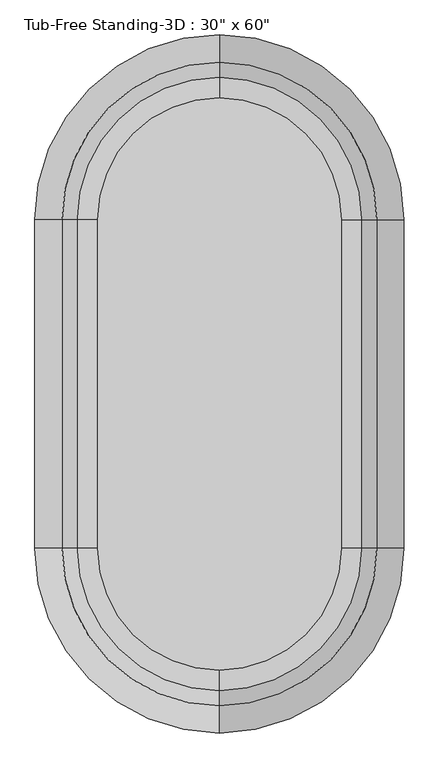
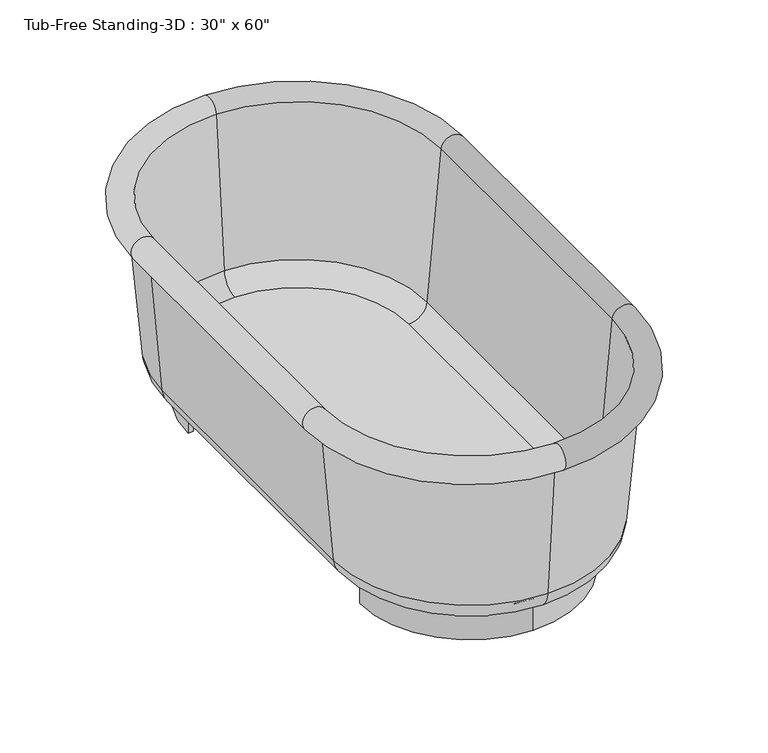
"""IFC4 building model written with IfcOpenShell, lengths in millimetres: flow terminal geometry."""

from ifc_helpers import new_model, si_unit, point, frame, frame_2d, origin, origin_with_axes, place, context, project, spatial, polyline, circle_curve, ellipse_curve, trimmed, segment, composite_curve, outline, extrude, source, transform, mapped, element, save
from ifc_brep_helpers import plane_surface, cylinder_surface, revolved_surface, advanced_brep


def flow_terminal_93af9e75(model_context):
    return source(origin(), model_context, "Body", "SolidModel", [
        extrude(outline(composite_curve([segment(trimmed(circle_curve(frame_2d((0.0, 304.8)), 215.9), [point((0.0, 520.7))], [point((-215.9, 304.8))], True, "CARTESIAN"), True, "CONTINUOUS"), segment(polyline([(-215.9, 304.8), (-226.1824236, 304.8)]), True, "CONTINUOUS"), segment(trimmed(circle_curve(frame_2d((0.0, 304.8)), 226.1824236), [point((-226.1824236, 304.8))], [point((0.0, 530.9824236))], False, "CARTESIAN"), True, "CONTINUOUS"), segment(trimmed(circle_curve(frame_2d((0.0, 304.8)), 226.1824236), [point((0.0, 530.9824236))], [point((226.1824236, 304.8))], False, "CARTESIAN"), True, "CONTINUOUS"), segment(polyline([(226.1824236, 304.8), (215.9, 304.8)]), True, "CONTINUOUS"), segment(trimmed(circle_curve(frame_2d((0.0, 304.8)), 215.9), [point((215.9, 304.8))], [point((0.0, 520.7))], True, "CARTESIAN"), True, "CONTINUOUS")], self_intersect=False)), origin_with_axes(), (0.0, 0.0, 1.0), 63.5),
        extrude(outline(composite_curve([segment(trimmed(circle_curve(frame_2d((0.0, -304.8)), 226.1824236), [point((0.0, -530.9824236))], [point((-226.1824236, -304.8))], False, "CARTESIAN"), True, "CONTINUOUS"), segment(polyline([(-226.1824236, -304.8), (-215.9, -304.8)]), True, "CONTINUOUS"), segment(trimmed(circle_curve(frame_2d((0.0, -304.8)), 215.9), [point((-215.9, -304.8))], [point((0.0, -520.7))], True, "CARTESIAN"), True, "CONTINUOUS"), segment(trimmed(circle_curve(frame_2d((0.0, -304.8)), 215.9), [point((0.0, -520.7))], [point((215.9, -304.8))], True, "CARTESIAN"), True, "CONTINUOUS"), segment(polyline([(215.9, -304.8), (226.1824236, -304.8)]), True, "CONTINUOUS"), segment(trimmed(circle_curve(frame_2d((0.0, -304.8)), 226.1824236), [point((226.1824236, -304.8))], [point((0.0, -530.9824236))], False, "CARTESIAN"), True, "CONTINUOUS")], self_intersect=False)), origin_with_axes(), (0.0, 0.0, 1.0), 63.5),
        extrude(outline(composite_curve([segment(polyline([(-226.1824236, -304.8), (-226.1824236, 304.8)]), True, "CONTINUOUS"), segment(trimmed(circle_curve(frame_2d((0.0, 304.8)), 226.1824236), [point((-226.1824236, 304.8))], [point((0.0, 530.9824236))], False, "CARTESIAN"), True, "CONTINUOUS"), segment(trimmed(circle_curve(frame_2d((0.0, 304.8)), 226.1824236), [point((0.0, 530.9824236))], [point((226.1824236, 304.8))], False, "CARTESIAN"), True, "CONTINUOUS"), segment(polyline([(226.1824236, 304.8), (226.1824236, -304.8)]), True, "CONTINUOUS"), segment(trimmed(circle_curve(frame_2d((0.0, -304.8)), 226.1824236), [point((226.1824236, -304.8))], [point((0.0, -530.9824236))], False, "CARTESIAN"), True, "CONTINUOUS"), segment(trimmed(circle_curve(frame_2d((0.0, -304.8)), 226.1824236), [point((0.0, -530.9824236))], [point((-226.1824236, -304.8))], False, "CARTESIAN"), True, "CONTINUOUS")], self_intersect=False)), frame((0.0, 0.0, 63.5), z_axis=(0.0, 0.0, 1.0), x_axis=(1.0, 0.0, 0.0)), (0.0, 0.0, 1.0), 15.08125),
        advanced_brep(
        [(0.0, -609.6, 406.4), (304.8, -304.8, 406.4), (317.5, -304.8, 406.4), (0.0, -622.3, 406.4), (0.0, -583.8045038, 111.5561295), (279.0045038, -304.8, 111.5561295), (0.0, -530.9824236, 63.1536107), (226.1824236, -304.8, 63.1536107), (0.0, -530.9824236, 78.0774627), (226.1824236, -304.8, 78.0774627), (0.0, -568.9374416, 112.8568289), (264.1374416, -304.8, 112.8568289), (0.0, -597.1561556, 435.3982063), (292.3561556, -304.8, 435.3982063), (-304.8, -304.8, 406.4), (-317.5, -304.8, 406.4), (-279.0045038, -304.8, 111.5561295), (-226.1824236, -304.8, 63.1536107), (-226.1824236, -304.8, 78.0774627), (-264.1374416, -304.8, 112.8568289), (-292.3561556, -304.8, 435.3982063), (-317.5, 304.8, 406.4), (-304.8, 304.8, 406.4), (-279.0045038, 304.8, 111.5561295), (-226.1824236, 304.8, 63.1536107), (-226.1824236, 304.8, 78.0774627), (-264.1374416, 304.8, 112.8568289), (-292.3561556, 304.8, 435.3982063), (0.0, 609.6, 406.4), (0.0, 622.3, 406.4), (0.0, 583.8045038, 111.5561295), (0.0, 530.9824236, 63.1536107), (0.0, 530.9824236, 78.0774627), (0.0, 568.9374416, 112.8568289), (0.0, 597.1561556, 435.3982063), (304.8, 304.8, 406.4), (317.5, 304.8, 406.4), (279.0045038, 304.8, 111.5561295), (226.1824236, 304.8, 63.1536107), (226.1824236, 304.8, 78.0774627), (264.1374416, 304.8, 112.8568289), (292.3561556, 304.8, 435.3982063)],
        [
            (0, 1, circle_curve(frame((0.0, -304.8, 406.4), z_axis=(0.0, 0.0, 1.0), x_axis=(1.0, 0.0, 0.0)), 304.8)),
            (1, 2),
            (2, 3, circle_curve(frame((0.0, -304.8, 406.4), z_axis=(0.0, 0.0, -1.0), x_axis=(1.0, 0.0, 0.0)), 317.5)),
            (3, 0),
            (4, 5, circle_curve(frame((0.0, -304.8, 111.5561295), z_axis=(0.0, 0.0, 1.0), x_axis=(1.0, 0.0, 0.0)), 279.0045038)),
            (5, 1),
            (0, 4),
            (6, 7, circle_curve(frame((0.0, -304.8, 63.1536107), z_axis=(0.0, 0.0, 1.0), x_axis=(1.0, 0.0, 0.0)), 226.1824236)),
            (7, 5, circle_curve(frame((226.1824236, -304.8, 116.1774627), z_axis=(0.0, -1.0, 0.0), x_axis=(1.0, 0.0, 0.0)), 53.023852)),
            (4, 6, circle_curve(frame((0.0, -530.9824236, 116.1774627), z_axis=(1.0, 0.0, 0.0), x_axis=(0.0, -1.0, 0.0)), 53.023852)),
            (8, 9, circle_curve(frame((0.0, -304.8, 78.0774627), z_axis=(0.0, 0.0, 1.0), x_axis=(1.0, 0.0, 0.0)), 226.1824236)),
            (9, 7),
            (6, 8),
            (10, 11, circle_curve(frame((0.0, -304.8, 112.8568289), z_axis=(0.0, 0.0, 1.0), x_axis=(1.0, 0.0, 0.0)), 264.1374416)),
            (11, 9, circle_curve(frame((226.1824236, -304.8, 116.1774627), z_axis=(0.0, 1.0, 0.0), x_axis=(1.0, 0.0, 0.0)), 38.1)),
            (8, 10, circle_curve(frame((0.0, -530.9824236, 116.1774627), z_axis=(-1.0, 0.0, 0.0), x_axis=(0.0, -1.0, 0.0)), 38.1)),
            (12, 13, circle_curve(frame((0.0, -304.8, 435.3982063), z_axis=(0.0, 0.0, 1.0), x_axis=(1.0, 0.0, 0.0)), 292.3561556)),
            (13, 11),
            (10, 12),
            (2, 13, circle_curve(frame((317.5, -304.8, 431.8), z_axis=(0.0, -1.0, 0.0), x_axis=(1.0, 0.0, 0.0)), 25.4)),
            (12, 3, circle_curve(frame((0.0, -622.3, 431.8), z_axis=(1.0, 0.0, 0.0), x_axis=(0.0, -1.0, 0.0)), 25.4)),
            (14, 0, circle_curve(frame((0.0, -304.8, 406.4), z_axis=(0.0, 0.0, 1.0), x_axis=(0.0, -1.0, 0.0)), 304.8)),
            (3, 15, circle_curve(frame((0.0, -304.8, 406.4), z_axis=(0.0, 0.0, -1.0), x_axis=(0.0, -1.0, 0.0)), 317.5)),
            (15, 14),
            (16, 4, circle_curve(frame((0.0, -304.8, 111.5561295), z_axis=(0.0, 0.0, 1.0), x_axis=(0.0, -1.0, 0.0)), 279.0045038)),
            (14, 16),
            (17, 6, circle_curve(frame((0.0, -304.8, 63.1536107), z_axis=(0.0, 0.0, 1.0), x_axis=(0.0, -1.0, 0.0)), 226.1824236)),
            (16, 17, circle_curve(frame((-226.1824236, -304.8, 116.1774627), z_axis=(0.0, -1.0, 0.0), x_axis=(-1.0, 0.0, 0.0)), 53.023852)),
            (18, 8, circle_curve(frame((0.0, -304.8, 78.0774627), z_axis=(0.0, 0.0, 1.0), x_axis=(0.0, -1.0, 0.0)), 226.1824236)),
            (17, 18),
            (19, 10, circle_curve(frame((0.0, -304.8, 112.8568289), z_axis=(0.0, 0.0, 1.0), x_axis=(0.0, -1.0, 0.0)), 264.1374416)),
            (18, 19, circle_curve(frame((-226.1824236, -304.8, 116.1774627), z_axis=(0.0, 1.0, 0.0), x_axis=(-1.0, 0.0, 0.0)), 38.1)),
            (20, 12, circle_curve(frame((0.0, -304.8, 435.3982063), z_axis=(0.0, 0.0, 1.0), x_axis=(0.0, -1.0, 0.0)), 292.3561556)),
            (19, 20),
            (20, 15, circle_curve(frame((-317.5, -304.8, 431.8), z_axis=(0.0, -1.0, 0.0), x_axis=(-1.0, 0.0, 0.0)), 25.4)),
            (15, 21),
            (21, 22),
            (22, 14),
            (22, 23),
            (23, 16),
            (23, 24, circle_curve(frame((-226.1824236, 304.8, 116.1774627), z_axis=(0.0, -1.0, 0.0), x_axis=(-1.0, 0.0, 0.0)), 53.023852)),
            (24, 17),
            (24, 25),
            (25, 18),
            (25, 26, circle_curve(frame((-226.1824236, 304.8, 116.1774627), z_axis=(0.0, 1.0, 0.0), x_axis=(-1.0, 0.0, 0.0)), 38.1)),
            (26, 19),
            (26, 27),
            (27, 20),
            (27, 21, circle_curve(frame((-317.5, 304.8, 431.8), z_axis=(0.0, -1.0, 0.0), x_axis=(-1.0, 0.0, 0.0)), 25.4)),
            (28, 22, circle_curve(frame((0.0, 304.8, 406.4), z_axis=(0.0, 0.0, 1.0), x_axis=(-1.0, 0.0, 0.0)), 304.8)),
            (21, 29, circle_curve(frame((0.0, 304.8, 406.4), z_axis=(0.0, 0.0, -1.0), x_axis=(-1.0, 0.0, 0.0)), 317.5)),
            (29, 28),
            (30, 23, circle_curve(frame((0.0, 304.8, 111.5561295), z_axis=(0.0, 0.0, 1.0), x_axis=(-1.0, 0.0, 0.0)), 279.0045038)),
            (28, 30),
            (31, 24, circle_curve(frame((0.0, 304.8, 63.1536107), z_axis=(0.0, 0.0, 1.0), x_axis=(-1.0, 0.0, 0.0)), 226.1824236)),
            (30, 31, circle_curve(frame((0.0, 530.9824236, 116.1774627), z_axis=(-1.0, 0.0, 0.0), x_axis=(0.0, 1.0, 0.0)), 53.023852)),
            (32, 25, circle_curve(frame((0.0, 304.8, 78.0774627), z_axis=(0.0, 0.0, 1.0), x_axis=(-1.0, 0.0, 0.0)), 226.1824236)),
            (31, 32),
            (33, 26, circle_curve(frame((0.0, 304.8, 112.8568289), z_axis=(0.0, 0.0, 1.0), x_axis=(-1.0, 0.0, 0.0)), 264.1374416)),
            (32, 33, circle_curve(frame((0.0, 530.9824236, 116.1774627), z_axis=(1.0, 0.0, 0.0), x_axis=(0.0, 1.0, 0.0)), 38.1)),
            (34, 27, circle_curve(frame((0.0, 304.8, 435.3982063), z_axis=(0.0, 0.0, 1.0), x_axis=(-1.0, 0.0, 0.0)), 292.3561556)),
            (33, 34),
            (34, 29, circle_curve(frame((0.0, 622.3, 431.8), z_axis=(-1.0, 0.0, 0.0), x_axis=(0.0, 1.0, 0.0)), 25.4)),
            (35, 28, circle_curve(frame((0.0, 304.8, 406.4), z_axis=(0.0, 0.0, 1.0), x_axis=(0.0, 1.0, 0.0)), 304.8)),
            (29, 36, circle_curve(frame((0.0, 304.8, 406.4), z_axis=(0.0, 0.0, -1.0), x_axis=(0.0, 1.0, 0.0)), 317.5)),
            (36, 35),
            (37, 30, circle_curve(frame((0.0, 304.8, 111.5561295), z_axis=(0.0, 0.0, 1.0), x_axis=(0.0, 1.0, 0.0)), 279.0045038)),
            (35, 37),
            (38, 31, circle_curve(frame((0.0, 304.8, 63.1536107), z_axis=(0.0, 0.0, 1.0), x_axis=(0.0, 1.0, 0.0)), 226.1824236)),
            (37, 38, circle_curve(frame((226.1824236, 304.8, 116.1774627), z_axis=(0.0, 1.0, 0.0), x_axis=(1.0, 0.0, 0.0)), 53.023852)),
            (39, 32, circle_curve(frame((0.0, 304.8, 78.0774627), z_axis=(0.0, 0.0, 1.0), x_axis=(0.0, 1.0, 0.0)), 226.1824236)),
            (38, 39),
            (40, 33, circle_curve(frame((0.0, 304.8, 112.8568289), z_axis=(0.0, 0.0, 1.0), x_axis=(0.0, 1.0, 0.0)), 264.1374416)),
            (39, 40, circle_curve(frame((226.1824236, 304.8, 116.1774627), z_axis=(0.0, -1.0, 0.0), x_axis=(1.0, 0.0, 0.0)), 38.1)),
            (41, 34, circle_curve(frame((0.0, 304.8, 435.3982063), z_axis=(0.0, 0.0, 1.0), x_axis=(0.0, 1.0, 0.0)), 292.3561556)),
            (40, 41),
            (41, 36, circle_curve(frame((317.5, 304.8, 431.8), z_axis=(0.0, 1.0, 0.0), x_axis=(1.0, 0.0, 0.0)), 25.4)),
            (36, 2),
            (1, 35),
            (5, 37),
            (7, 38),
            (9, 39),
            (11, 40),
            (13, 41),
        ],
        [
            plane_surface(frame((0.0, -304.8, 406.4), z_axis=(0.0, 0.0, -1.0), x_axis=(1.0, 0.0, 0.0))),
            revolved_surface(polyline([(304.8, -304.8, 406.4), (279.0045038, -304.8, 111.5561295)]), (0.0, -304.8, 431.8), (0.0, 0.0, -1.0)),
            revolved_surface(trimmed(ellipse_curve(frame((226.1824236, -304.8, 116.1774627), z_axis=(0.0, 1.0, 0.0), x_axis=(1.0, 0.0, 0.0)), 53.023852, 53.023852), [point((279.0045038, -304.8, 111.5561295))], [point((226.1824236, -304.8, 63.1536107))], True, "CARTESIAN"), (0.0, -304.8, 431.8), (0.0, 0.0, -1.0)),
            revolved_surface(polyline([(226.1824236, -304.8, 63.1536107), (226.1824236, -304.8, 78.07746270000001)]), (0.0, -304.8, 431.8), (0.0, 0.0, -1.0)),
            revolved_surface(trimmed(ellipse_curve(frame((226.1824236, -304.8, 116.1774627), z_axis=(0.0, -1.0, 0.0), x_axis=(1.0, 0.0, 0.0)), 38.1, 38.1), [point((226.1824236, -304.8, 78.0774627))], [point((264.1374416, -304.8, 112.8568289))], True, "CARTESIAN"), (0.0, -304.8, 431.8), (0.0, 0.0, -1.0)),
            revolved_surface(polyline([(264.1374416, -304.8, 112.8568289), (292.3561556, -304.8, 435.3982063)]), (0.0, -304.8, 431.8), (0.0, 0.0, -1.0)),
            revolved_surface(trimmed(ellipse_curve(frame((317.5, -304.8, 431.8), z_axis=(0.0, 1.0, 0.0), x_axis=(1.0, 0.0, 0.0)), 25.4, 25.4), [point((292.3561556, -304.8, 435.3982063))], [point((317.5, -304.8, 406.4))], True, "CARTESIAN"), (0.0, -304.8, 431.8), (0.0, 0.0, -1.0)),
            plane_surface(frame((0.0, -304.8, 406.4), z_axis=(0.0, 0.0, -1.0), x_axis=(0.0, -1.0, 0.0))),
            revolved_surface(polyline([(0.0, -609.6, 406.4), (0.0, -583.8045038, 111.5561295)]), (0.0, -304.8, 431.8), (0.0, 0.0, -1.0)),
            revolved_surface(trimmed(ellipse_curve(frame((0.0, -530.9824236, 116.1774627), z_axis=(1.0, 0.0, 0.0), x_axis=(0.0, -1.0, 0.0)), 53.023852, 53.023852), [point((0.0, -583.8045038, 111.5561295))], [point((0.0, -530.9824236, 63.1536107))], True, "CARTESIAN"), (0.0, -304.8, 431.8), (0.0, 0.0, -1.0)),
            revolved_surface(polyline([(0.0, -530.9824236, 63.1536107), (0.0, -530.9824236, 78.07746270000001)]), (0.0, -304.8, 431.8), (0.0, 0.0, -1.0)),
            revolved_surface(trimmed(ellipse_curve(frame((0.0, -530.9824236, 116.1774627), z_axis=(-1.0, 0.0, 0.0), x_axis=(0.0, -1.0, 0.0)), 38.1, 38.1), [point((0.0, -530.9824236, 78.0774627))], [point((0.0, -568.9374416, 112.8568289))], True, "CARTESIAN"), (0.0, -304.8, 431.8), (0.0, 0.0, -1.0)),
            revolved_surface(polyline([(0.0, -568.9374416, 112.8568289), (0.0, -597.1561556, 435.3982063)]), (0.0, -304.8, 431.8), (0.0, 0.0, -1.0)),
            revolved_surface(trimmed(ellipse_curve(frame((0.0, -622.3, 431.8), z_axis=(1.0, 0.0, 0.0), x_axis=(0.0, -1.0, 0.0)), 25.4, 25.4), [point((0.0, -597.1561556, 435.3982063))], [point((0.0, -622.3, 406.4))], True, "CARTESIAN"), (0.0, -304.8, 431.8), (0.0, 0.0, -1.0)),
            plane_surface(frame((-317.5, -304.8, 406.4), z_axis=(0.0, 0.0, -1.0), x_axis=(0.0, 1.0, 0.0))),
            plane_surface(frame((-304.8, -304.8, 406.4), z_axis=(-0.9961946980917455, 0.0, -0.08715574274765882), x_axis=(0.0, 1.0, 0.0))),
            cylinder_surface(frame((-226.1824236, -304.8, 116.1774627), z_axis=(0.0, -1.0, 0.0), x_axis=(-1.0, 0.0, 0.0)), 53.023852),
            plane_surface(frame((-226.1824236, -304.8, 63.1536107), z_axis=(1.0, 0.0, 0.0), x_axis=(0.0, 1.0, 0.0))),
            revolved_surface(polyline([(-264.2824236, 304.8, 116.1774627), (-264.2824236, -304.8, 116.1774627)]), (-226.1824236, -304.8, 116.1774627), (0.0, 1.0, 0.0)),
            plane_surface(frame((-264.1374416, -304.8, 112.8568289), z_axis=(0.9961946980917457, 0.0, 0.08715574274765679), x_axis=(0.0, 1.0, 0.0))),
            cylinder_surface(frame((-317.5, -304.8, 431.8), z_axis=(0.0, -1.0, 0.0), x_axis=(-1.0, 0.0, 0.0)), 25.4),
            plane_surface(frame((0.0, 304.8, 406.4), z_axis=(0.0, 0.0, -1.0), x_axis=(-1.0, 0.0, 0.0))),
            revolved_surface(polyline([(-304.8, 304.8, 406.4), (-279.0045038, 304.8, 111.5561295)]), (0.0, 304.8, 431.8), (0.0, 0.0, -1.0)),
            revolved_surface(trimmed(ellipse_curve(frame((-226.1824236, 304.8, 116.1774627), z_axis=(0.0, -1.0, 0.0), x_axis=(-1.0, 0.0, 0.0)), 53.023852, 53.023852), [point((-279.0045038, 304.8, 111.5561295))], [point((-226.1824236, 304.8, 63.1536107))], True, "CARTESIAN"), (0.0, 304.8, 431.8), (0.0, 0.0, -1.0)),
            revolved_surface(polyline([(-226.1824236, 304.8, 63.1536107), (-226.1824236, 304.8, 78.07746270000001)]), (0.0, 304.8, 431.8), (0.0, 0.0, -1.0)),
            revolved_surface(trimmed(ellipse_curve(frame((-226.1824236, 304.8, 116.1774627), z_axis=(0.0, 1.0, 0.0), x_axis=(-1.0, 0.0, 0.0)), 38.1, 38.1), [point((-226.1824236, 304.8, 78.0774627))], [point((-264.1374416, 304.8, 112.8568289))], True, "CARTESIAN"), (0.0, 304.8, 431.8), (0.0, 0.0, -1.0)),
            revolved_surface(polyline([(-264.1374416, 304.8, 112.8568289), (-292.3561556, 304.8, 435.3982063)]), (0.0, 304.8, 431.8), (0.0, 0.0, -1.0)),
            revolved_surface(trimmed(ellipse_curve(frame((-317.5, 304.8, 431.8), z_axis=(0.0, -1.0, 0.0), x_axis=(-1.0, 0.0, 0.0)), 25.4, 25.4), [point((-292.3561556, 304.8, 435.3982063))], [point((-317.5, 304.8, 406.4))], True, "CARTESIAN"), (0.0, 304.8, 431.8), (0.0, 0.0, -1.0)),
            plane_surface(frame((0.0, 304.8, 406.4), z_axis=(0.0, 0.0, -1.0), x_axis=(0.0, 1.0, 0.0))),
            revolved_surface(polyline([(0.0, 609.6, 406.4), (0.0, 583.8045038, 111.5561295)]), (0.0, 304.8, 431.8), (0.0, 0.0, -1.0)),
            revolved_surface(trimmed(ellipse_curve(frame((0.0, 530.9824236, 116.1774627), z_axis=(-1.0, 0.0, 0.0), x_axis=(0.0, 1.0, 0.0)), 53.023852, 53.023852), [point((0.0, 583.8045038, 111.5561295))], [point((0.0, 530.9824236, 63.1536107))], True, "CARTESIAN"), (0.0, 304.8, 431.8), (0.0, 0.0, -1.0)),
            revolved_surface(polyline([(0.0, 530.9824236, 63.1536107), (0.0, 530.9824236, 78.07746270000001)]), (0.0, 304.8, 431.8), (0.0, 0.0, -1.0)),
            revolved_surface(trimmed(ellipse_curve(frame((0.0, 530.9824236, 116.1774627), z_axis=(1.0, 0.0, 0.0), x_axis=(0.0, 1.0, 0.0)), 38.1, 38.1), [point((0.0, 530.9824236, 78.0774627))], [point((0.0, 568.9374416, 112.8568289))], True, "CARTESIAN"), (0.0, 304.8, 431.8), (0.0, 0.0, -1.0)),
            revolved_surface(polyline([(0.0, 568.9374416, 112.8568289), (0.0, 597.1561556, 435.3982063)]), (0.0, 304.8, 431.8), (0.0, 0.0, -1.0)),
            revolved_surface(trimmed(ellipse_curve(frame((0.0, 622.3, 431.8), z_axis=(-1.0, 0.0, 0.0), x_axis=(0.0, 1.0, 0.0)), 25.4, 25.4), [point((0.0, 597.1561556, 435.3982063))], [point((0.0, 622.3, 406.4))], True, "CARTESIAN"), (0.0, 304.8, 431.8), (0.0, 0.0, -1.0)),
            plane_surface(frame((317.5, 304.8, 406.4), z_axis=(0.0, 0.0, -1.0), x_axis=(0.0, -1.0, 0.0))),
            plane_surface(frame((304.8, 304.8, 406.4), z_axis=(0.9961946980917455, 0.0, -0.08715574274765882), x_axis=(0.0, -1.0, 0.0))),
            cylinder_surface(frame((226.1824236, 304.8, 116.1774627), z_axis=(0.0, 1.0, 0.0), x_axis=(1.0, 0.0, 0.0)), 53.023852),
            plane_surface(frame((226.1824236, 304.8, 63.1536107), z_axis=(-1.0, 0.0, 0.0), x_axis=(0.0, -1.0, 0.0))),
            revolved_surface(polyline([(264.2824236, -304.8, 116.1774627), (264.2824236, 304.8, 116.1774627)]), (226.1824236, 304.8, 116.1774627), (0.0, -1.0, 0.0)),
            plane_surface(frame((264.1374416, 304.8, 112.8568289), z_axis=(-0.9961946980917458, 0.0, 0.0871557427476568), x_axis=(0.0, -1.0, 0.0))),
            cylinder_surface(frame((317.5, 304.8, 431.8), z_axis=(0.0, 1.0, 0.0), x_axis=(1.0, 0.0, 0.0)), 25.4),
        ],
        [
            (0, [[1, 2, 3, 4]]),
            (1, [[5, 6, -1, 7]]),
            (2, [[8, 9, -5, 10]]),
            (3, [[11, 12, -8, 13]]),
            (4, [[14, 15, -11, 16]]),
            (5, [[17, 18, -14, 19]]),
            (6, [[-3, 20, -17, 21]]),
            (7, [[22, -4, 23, 24]]),
            (8, [[25, -7, -22, 26]]),
            (9, [[27, -10, -25, 28]]),
            (10, [[29, -13, -27, 30]]),
            (11, [[31, -16, -29, 32]]),
            (12, [[33, -19, -31, 34]]),
            (13, [[-23, -21, -33, 35]]),
            (14, [[-24, 36, 37, 38]]),
            (15, [[-26, -38, 39, 40]]),
            (16, [[-28, -40, 41, 42]]),
            (17, [[-30, -42, 43, 44]]),
            (18, [[-32, -44, 45, 46]]),
            (19, [[-34, -46, 47, 48]]),
            (20, [[-35, -48, 49, -36]]),
            (21, [[50, -37, 51, 52]]),
            (22, [[53, -39, -50, 54]]),
            (23, [[55, -41, -53, 56]]),
            (24, [[57, -43, -55, 58]]),
            (25, [[59, -45, -57, 60]]),
            (26, [[61, -47, -59, 62]]),
            (27, [[-51, -49, -61, 63]]),
            (28, [[64, -52, 65, 66]]),
            (29, [[67, -54, -64, 68]]),
            (30, [[69, -56, -67, 70]]),
            (31, [[71, -58, -69, 72]]),
            (32, [[73, -60, -71, 74]]),
            (33, [[75, -62, -73, 76]]),
            (34, [[-65, -63, -75, 77]]),
            (35, [[-66, 78, -2, 79]]),
            (36, [[-68, -79, -6, 80]]),
            (37, [[-70, -80, -9, 81]]),
            (38, [[-72, -81, -12, 82]]),
            (39, [[-74, -82, -15, 83]]),
            (40, [[-76, -83, -18, 84]]),
            (41, [[-77, -84, -20, -78]]),
        ],
    ),
    ])


if __name__ == "__main__":
    model = new_model("IFC4")
    model_context = context("Model", 3, world=origin())
    ifc_project = project(units=[si_unit("LENGTHUNIT", "METRE", prefix="MILLI")], contexts=[model_context])
    site = spatial("IfcSite", under=ifc_project)
    building = spatial("IfcBuilding", under=site)
    placement = place(None, origin())
    flow_terminal_shape = flow_terminal_93af9e75(model_context)
    element("IfcFlowTerminal", 1, ObjectType="Tub-Free Standing-3D : 30\" x 60\"", at=placement, inside=building, context=model_context, shape_type="MappedRepresentation", body=[
        mapped(flow_terminal_shape, transform((0.0, 0.0, 0.0), x_axis=(1.0, 0.0, 0.0), y_axis=(0.0, 1.0, 0.0), z_axis=(0.0, 0.0, 1.0))),
    ])
    save(model, "model.ifc")

# Revit data of these elements
# Type "Tub-Free Standing-3D : 30\" x 60\""
#   Assembly Code = "D2010110"
#   Height = 1' - 6"
#   Length = 4' - 3"
#   Width = 2' - 3"
#   Tub Material = Porcelain, Ivory
#   Default Elevation = 0
# Element 1 (IfcFlowTerminal, "Tub-Free Standing-3D : 30\" x 60\"")
#   Materials on its faces: "Porcelain, Ivory"
# Materials
#   "Porcelain, Ivory": class "Ceramic", colour RGB 247 247 239, transparency 0, Description = "Porcelain, ivory", Cost = 0
